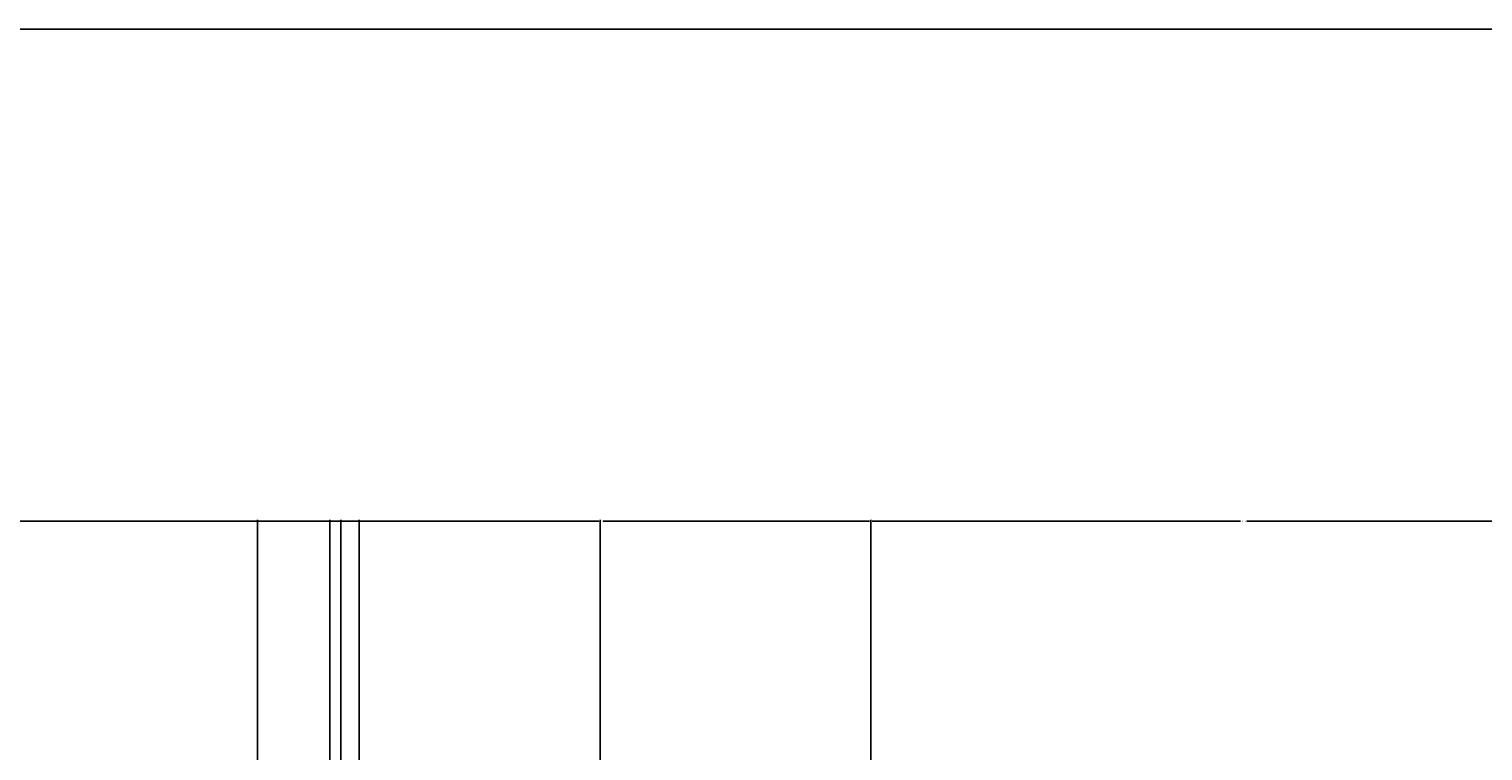
# Model space of a CAD drawing. Units: inches. Extents: x 1965 to 2673, y 1802 to 2669.
# Tile 12 of 16: x 2168 to 2372, y 2568 to 2669. Entities that reach past the tile are written whole.
import ezdxf

# ---------------------------------------------------------------- set-up
doc = ezdxf.new("R2010")
doc.units = ezdxf.units.IN
doc.layers.add('A-ANNO-DIMS', color=2, linetype='Continuous', lineweight=18)
doc.layers.add('A-ANNO-TTLB', color=7, linetype='Continuous', lineweight=25)
doc.styles.get("Standard").update_dxf_attribs({"font": 'arial.ttf'})
doc.dimstyles.get("Standard").update_dxf_attribs({"dimtxt": 0.18, "dimasz": 0.18, "dimexe": 0.18, "dimexo": 0.0625, "dimgap": 0.09, "dimtad": 0, "dimtih": 1, "dimtoh": 1, "dimdec": 4, "dimzin": 0, "dimdsep": 46, "dimtxsty": 'Standard', "dimcen": 0.09, "dimadec": 0, "dimazin": 0, "dimtfac": 1, "dimtdec": 4, "dimtofl": 0, "dimtmove": 0, "dimatfit": 3, "dimfxl": 1, "dimtolj": 1, "dimtzin": 0, "dimarcsym": 0})

# ---------------------------------------------------------------- blocks, each defined once
blk = doc.blocks.new('*D28')
at = {"layer": 'A-ANNO-DIMS', "color": 0, "lineweight": -2, "transparency": 16777216}
for p, q in [((2076.76, 2565.65), (2076.76, 2600.5)), ((2076.94, 2600.32), (2143.04, 2600.32)), ((2210.05, 2600.32), (2143.95, 2600.32)), ((2210.23, 2565.65), (2210.23, 2600.5))]:
    blk.add_line(p, q, dxfattribs=at)
at = {"layer": 'A-ANNO-DIMS', "color": 0, "transparency": 16777216}
for points in [[(2076.94, 2600.35), (2076.94, 2600.29), (2076.76, 2600.32)], [(2210.05, 2600.35), (2210.05, 2600.29), (2210.23, 2600.32)]]:
    blk.add_solid(points, dxfattribs=at)
at = {"layer": 'Defpoints', "color": 0, "transparency": 16777216}
for p in [(2210.23, 2600.32), (2076.76, 2565.59), (2210.23, 2565.59)]:
    blk.add_point(p, dxfattribs=at)
at = {"layer": 'A-ANNO-DIMS', "color": 0, "transparency": 16777216, "insert": (2143.49, 2600.32), "char_height": 0.18, "attachment_point": 5}
blk.add_mtext('\\A1;133.48', dxfattribs=at)
blk = doc.blocks.new('*D29')
at = {"layer": 'A-ANNO-DIMS', "color": 0, "lineweight": -2, "transparency": 16777216}
for p, q in [((2210.23, 2565.65), (2210.23, 2600.5)), ((2210.41, 2600.32), (2247.71, 2600.32)), ((2285.79, 2600.32), (2248.5, 2600.32)), ((2285.97, 2565.65), (2285.97, 2600.5))]:
    blk.add_line(p, q, dxfattribs=at)
at = {"layer": 'A-ANNO-DIMS', "color": 0, "transparency": 16777216}
for points in [[(2210.41, 2600.35), (2210.41, 2600.29), (2210.23, 2600.32)], [(2285.79, 2600.35), (2285.79, 2600.29), (2285.97, 2600.32)]]:
    blk.add_solid(points, dxfattribs=at)
at = {"layer": 'Defpoints', "color": 0, "transparency": 16777216}
for p in [(2285.97, 2600.32), (2210.23, 2565.59), (2285.97, 2565.59)]:
    blk.add_point(p, dxfattribs=at)
at = {"layer": 'A-ANNO-DIMS', "color": 0, "transparency": 16777216, "insert": (2248.1, 2600.32), "char_height": 0.18, "attachment_point": 5}
blk.add_mtext('\\A1;75.74', dxfattribs=at)
blk = doc.blocks.new('*D30')
at = {"layer": 'A-ANNO-DIMS', "color": 0, "lineweight": -2, "transparency": 16777216}
for p, q in [((2285.97, 2565.65), (2285.97, 2600.5)), ((2286.15, 2600.32), (2337.74, 2600.32)), ((2390.24, 2600.32), (2338.65, 2600.32)), ((2390.42, 2565.65), (2390.42, 2600.5))]:
    blk.add_line(p, q, dxfattribs=at)
at = {"layer": 'A-ANNO-DIMS', "color": 0, "transparency": 16777216}
for points in [[(2286.15, 2600.35), (2286.15, 2600.29), (2285.97, 2600.32)], [(2390.24, 2600.35), (2390.24, 2600.29), (2390.42, 2600.32)]]:
    blk.add_solid(points, dxfattribs=at)
at = {"layer": 'Defpoints', "color": 0, "transparency": 16777216}
for p in [(2390.42, 2600.32), (2285.97, 2565.59), (2390.42, 2565.59)]:
    blk.add_point(p, dxfattribs=at)
at = {"layer": 'A-ANNO-DIMS', "color": 0, "transparency": 16777216, "insert": (2338.2, 2600.32), "char_height": 0.18, "attachment_point": 5}
blk.add_mtext('\\A1;104.44', dxfattribs=at)
blk = doc.blocks.new('*D40')
at = {"layer": 'A-ANNO-DIMS', "color": 0, "lineweight": -2, "transparency": 16777216}
for p, q in [((2200.09, 1936.15), (2200.09, 2600.5)), ((2200.27, 2600.32), (2205.48, 2600.32)), ((2211.59, 2600.32), (2206.38, 2600.32)), ((2211.77, 1936.15), (2211.77, 2600.5))]:
    blk.add_line(p, q, dxfattribs=at)
at = {"layer": 'A-ANNO-DIMS', "color": 0, "transparency": 16777216}
for points in [[(2200.27, 2600.35), (2200.27, 2600.29), (2200.09, 2600.32)], [(2211.59, 2600.35), (2211.59, 2600.29), (2211.77, 2600.32)]]:
    blk.add_solid(points, dxfattribs=at)
at = {"layer": 'Defpoints', "color": 0, "transparency": 16777216}
for p in [(2211.77, 2600.32), (2200.09, 1936.09), (2211.77, 1936.09)]:
    blk.add_point(p, dxfattribs=at)
at = {"layer": 'A-ANNO-DIMS', "color": 0, "transparency": 16777216, "insert": (2205.93, 2600.32), "char_height": 0.18, "attachment_point": 5}
blk.add_mtext('\\A1;11.674', dxfattribs=at)
blk = doc.blocks.new('*D52')
at = {"layer": 'A-ANNO-DIMS', "color": 0, "lineweight": -2, "transparency": 16777216}
for p, q in [((2214.34, 2423.1), (2214.34, 2600.5)), ((2214.52, 2600.32), (2230.82, 2600.32)), ((2247.91, 2600.32), (2231.61, 2600.32)), ((2248.09, 2423.1), (2248.09, 2600.5))]:
    blk.add_line(p, q, dxfattribs=at)
at = {"layer": 'A-ANNO-DIMS', "color": 0, "transparency": 16777216}
for points in [[(2214.52, 2600.35), (2214.52, 2600.29), (2214.34, 2600.32)], [(2247.91, 2600.35), (2247.91, 2600.29), (2248.09, 2600.32)]]:
    blk.add_solid(points, dxfattribs=at)
at = {"layer": 'Defpoints', "color": 0, "transparency": 16777216}
for p in [(2248.09, 2600.32), (2214.34, 2423.04), (2248.09, 2423.04)]:
    blk.add_point(p, dxfattribs=at)
at = {"layer": 'A-ANNO-DIMS', "color": 0, "transparency": 16777216, "insert": (2231.22, 2600.32), "char_height": 0.18, "attachment_point": 5}
blk.add_mtext('\\A1;33.75', dxfattribs=at)

msp = doc.modelspace()

# ---------------------------------------------------------------- linework, layer by layer
at = {"layer": 'A-ANNO-TTLB'}
msp.add_lwpolyline([(1964.5703, 2669.282), (2673.2605, 2669.282), (2673.2605, 1802.0221), (1964.5703, 1802.0221)], close=True, dxfattribs=at)

# ---------------------------------------------------------------- dimensions: what is measured, and where the dimension line sits
at = {"layer": 'A-ANNO-DIMS'}
for base, p1, p2, override, picture, middle in [((2210.2316, 2600.3164), (2076.7559, 2565.5914), (2210.2316, 2565.5914), {"dimdec": 2, "dimlfac": 1, "dimrnd": 0, "dimzin": 0, "dimdsep": 46, "dimlunit": 2}, '*D28', (2143.4937, 2600.3164)), ((2211.767, 2600.3164), (2200.0927, 1936.0914), (2211.767, 1936.0914), {"dimdec": 3, "dimlfac": 1, "dimrnd": 0, "dimzin": 0, "dimdsep": 46, "dimlunit": 2}, '*D40', (2205.9299, 2600.3164)), ((2285.9734, 2600.3164), (2210.2316, 2565.5914), (2285.9734, 2565.5914), {"dimdec": 2, "dimlfac": 1, "dimrnd": 0, "dimzin": 0, "dimdsep": 46, "dimlunit": 2}, '*D29', (2248.1025, 2600.3164)), ((2248.0927, 2600.3164), (2214.3427, 2423.0404), (2248.0927, 2423.0404), {"dimdec": 2, "dimlfac": 1, "dimrnd": 0, "dimzin": 0, "dimdsep": 46, "dimlunit": 2}, '*D52', (2231.2177, 2600.3164)), ((2390.4173, 2600.3164), (2285.9734, 2565.5914), (2390.4173, 2565.5914), {"dimdec": 2, "dimlfac": 1, "dimrnd": 0, "dimzin": 0, "dimdsep": 46, "dimlunit": 2}, '*D30', (2338.1953, 2600.3164))]:
    dim = msp.add_linear_dim(base=base, p1=p1, p2=p2, dimstyle='Standard', override=override, dxfattribs=at)
    dim.commit()
    dim.dimension.update_dxf_attribs({"geometry": picture, "text_midpoint": middle})

doc.saveas('drawing.dxf')
